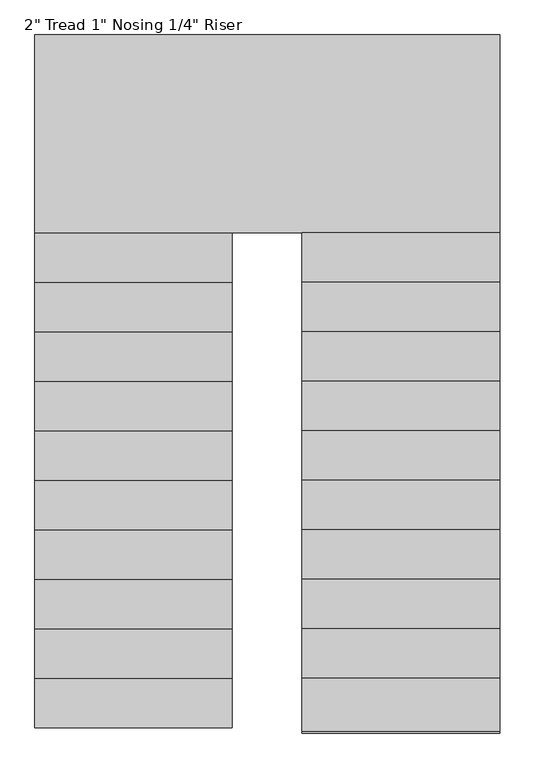
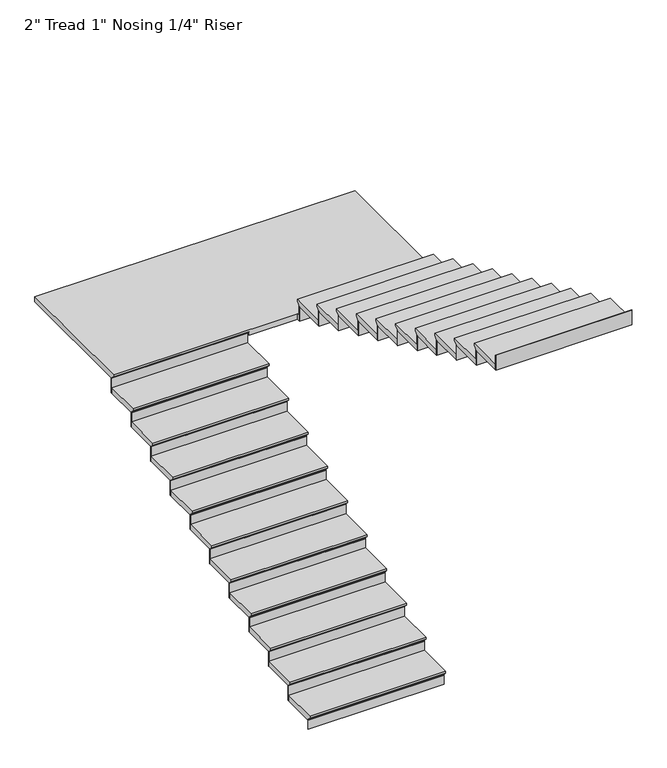
"""IFC4 building model written with IfcOpenShell, lengths in millimetres: stair flight geometry."""

from ifc_helpers import new_model, si_unit, origin, place, context, project, spatial, faceted_brep, source, transform, mapped, element, save


def stair_flight_447a52d2(model_context):
    return source(origin(), model_context, "Body", "Brep", [
        faceted_brep([(-629.5987998, 3364.6067329, 25722.6954545), (-629.5987998, 3364.6067329, 25741.7454545), (-1845.5417538, 3364.6067329, 25741.7454545), (-1845.5417538, 3364.6067329, 25722.6954545), (-629.5987998, 3390.0067329, 25697.2954545), (-1845.5417538, 3390.0067329, 25697.2954545), (-629.5987998, 3694.8067329, 25741.7454545), (-1845.5417538, 3694.8067329, 25741.7454545), (-1845.5417538, 3390.0067329, 25690.9454545), (-1845.5417538, 3694.8067329, 25690.9454545), (-629.5987998, 3694.8067329, 25690.9454545), (-629.5987998, 3390.0067329, 25690.9454545)], [[[0, 1, 2, 3]], [[4, 0, 3, 5]], [[2, 1, 6, 7]], [[8, 9, 10, 11]], [[2, 7, 9, 8, 5, 3]], [[8, 11, 4, 5]], [[6, 1, 0, 4, 11, 10]], [[7, 6, 10, 9]]]),
        faceted_brep([(-629.5987998, 3390.0067329, 25690.9454545), (-629.5987998, 3390.0067329, 25603.2), (-629.5987998, 3396.3567329, 25603.2), (-629.5987998, 3396.3567329, 25690.9454545), (-1845.5417538, 3390.0067329, 25690.9454545), (-1845.5417538, 3396.3567329, 25690.9454545), (-1845.5417538, 3396.3567329, 25603.2), (-1845.5417538, 3390.0067329, 25603.2)], [[[0, 1, 2, 3]], [[4, 5, 6, 7]], [[1, 0, 4, 7]], [[2, 1, 7, 6]], [[3, 2, 6, 5]], [[0, 3, 5, 4]]]),
        faceted_brep([(-629.5987998, 3694.8067329, 25829.4909091), (-629.5987998, 3694.8067329, 25690.9454545), (-629.5987998, 3701.1567329, 25690.9454545), (-629.5987998, 3701.1567329, 25829.4909091), (-1845.5417538, 3694.8067329, 25829.4909091), (-1845.5417538, 3701.1567329, 25829.4909091), (-1845.5417538, 3701.1567329, 25690.9454545), (-1845.5417538, 3694.8067329, 25690.9454545)], [[[0, 1, 2, 3]], [[4, 5, 6, 7]], [[1, 0, 4, 7]], [[2, 1, 7, 6]], [[3, 2, 6, 5]], [[0, 3, 5, 4]]]),
        faceted_brep([(-1845.5417538, 3669.4067329, 25880.2909091), (-629.5987998, 3669.4067329, 25880.2909091), (-629.5987998, 3999.6067329, 25880.2909091), (-1845.5417538, 3999.6067329, 25880.2909091), (-1845.5417538, 3694.8067329, 25829.4909091), (-1845.5417538, 3999.6067329, 25829.4909091), (-629.5987998, 3999.6067329, 25829.4909091), (-629.5987998, 3694.8067329, 25829.4909091), (-1845.5417538, 3694.8067329, 25835.8409091), (-1845.5417538, 3669.4067329, 25861.2409091), (-629.5987998, 3694.8067329, 25835.8409091), (-629.5987998, 3669.4067329, 25861.2409091)], [[[0, 1, 2, 3]], [[4, 5, 6, 7]], [[0, 3, 5, 4, 8, 9]], [[4, 7, 10, 8]], [[2, 1, 11, 10, 7, 6]], [[3, 2, 6, 5]], [[11, 1, 0, 9]], [[10, 11, 9, 8]]]),
        faceted_brep([(-629.5987998, 3999.6067329, 25968.0363636), (-629.5987998, 3999.6067329, 25829.4909091), (-629.5987998, 4005.9567329, 25829.4909091), (-629.5987998, 4005.9567329, 25968.0363636), (-1845.5417538, 3999.6067329, 25968.0363636), (-1845.5417538, 4005.9567329, 25968.0363636), (-1845.5417538, 4005.9567329, 25829.4909091), (-1845.5417538, 3999.6067329, 25829.4909091)], [[[0, 1, 2, 3]], [[4, 5, 6, 7]], [[1, 0, 4, 7]], [[2, 1, 7, 6]], [[3, 2, 6, 5]], [[0, 3, 5, 4]]]),
        faceted_brep([(-1845.5417538, 3974.2067329, 26018.8363636), (-629.5987998, 3974.2067329, 26018.8363636), (-629.5987998, 4304.4067329, 26018.8363636), (-1845.5417538, 4304.4067329, 26018.8363636), (-1845.5417538, 3999.6067329, 25968.0363636), (-1845.5417538, 4304.4067329, 25968.0363636), (-629.5987998, 4304.4067329, 25968.0363636), (-629.5987998, 3999.6067329, 25968.0363636), (-1845.5417538, 3999.6067329, 25974.3863636), (-1845.5417538, 3974.2067329, 25999.7863636), (-629.5987998, 3999.6067329, 25974.3863636), (-629.5987998, 3974.2067329, 25999.7863636)], [[[0, 1, 2, 3]], [[4, 5, 6, 7]], [[0, 3, 5, 4, 8, 9]], [[4, 7, 10, 8]], [[2, 1, 11, 10, 7, 6]], [[3, 2, 6, 5]], [[11, 1, 0, 9]], [[10, 11, 9, 8]]]),
        faceted_brep([(-629.5987998, 4304.4067329, 26106.5818182), (-629.5987998, 4304.4067329, 25968.0363636), (-629.5987998, 4310.7567329, 25968.0363636), (-629.5987998, 4310.7567329, 26106.5818182), (-1845.5417538, 4304.4067329, 26106.5818182), (-1845.5417538, 4310.7567329, 26106.5818182), (-1845.5417538, 4310.7567329, 25968.0363636), (-1845.5417538, 4304.4067329, 25968.0363636)], [[[0, 1, 2, 3]], [[4, 5, 6, 7]], [[1, 0, 4, 7]], [[2, 1, 7, 6]], [[3, 2, 6, 5]], [[0, 3, 5, 4]]]),
        faceted_brep([(-1845.5417538, 4279.0067329, 26157.3818182), (-629.5987998, 4279.0067329, 26157.3818182), (-629.5987998, 4609.2067329, 26157.3818182), (-1845.5417538, 4609.2067329, 26157.3818182), (-1845.5417538, 4304.4067329, 26106.5818182), (-1845.5417538, 4609.2067329, 26106.5818182), (-629.5987998, 4609.2067329, 26106.5818182), (-629.5987998, 4304.4067329, 26106.5818182), (-1845.5417538, 4304.4067329, 26112.9318182), (-1845.5417538, 4279.0067329, 26138.3318182), (-629.5987998, 4304.4067329, 26112.9318182), (-629.5987998, 4279.0067329, 26138.3318182)], [[[0, 1, 2, 3]], [[4, 5, 6, 7]], [[0, 3, 5, 4, 8, 9]], [[4, 7, 10, 8]], [[2, 1, 11, 10, 7, 6]], [[3, 2, 6, 5]], [[11, 1, 0, 9]], [[10, 11, 9, 8]]]),
        faceted_brep([(-629.5987998, 4609.2067329, 26245.1272727), (-629.5987998, 4609.2067329, 26106.5818182), (-629.5987998, 4615.5567329, 26106.5818182), (-629.5987998, 4615.5567329, 26245.1272727), (-1845.5417538, 4609.2067329, 26245.1272727), (-1845.5417538, 4615.5567329, 26245.1272727), (-1845.5417538, 4615.5567329, 26106.5818182), (-1845.5417538, 4609.2067329, 26106.5818182)], [[[0, 1, 2, 3]], [[4, 5, 6, 7]], [[1, 0, 4, 7]], [[2, 1, 7, 6]], [[3, 2, 6, 5]], [[0, 3, 5, 4]]]),
        faceted_brep([(-1845.5417538, 4583.8067329, 26295.9272727), (-629.5987998, 4583.8067329, 26295.9272727), (-629.5987998, 4914.0067329, 26295.9272727), (-1845.5417538, 4914.0067329, 26295.9272727), (-1845.5417538, 4609.2067329, 26245.1272727), (-1845.5417538, 4914.0067329, 26245.1272727), (-629.5987998, 4914.0067329, 26245.1272727), (-629.5987998, 4609.2067329, 26245.1272727), (-1845.5417538, 4609.2067329, 26251.4772727), (-1845.5417538, 4583.8067329, 26276.8772727), (-629.5987998, 4609.2067329, 26251.4772727), (-629.5987998, 4583.8067329, 26276.8772727)], [[[0, 1, 2, 3]], [[4, 5, 6, 7]], [[0, 3, 5, 4, 8, 9]], [[4, 7, 10, 8]], [[2, 1, 11, 10, 7, 6]], [[3, 2, 6, 5]], [[11, 1, 0, 9]], [[10, 11, 9, 8]]]),
        faceted_brep([(-629.5987998, 4914.0067329, 26383.6727273), (-629.5987998, 4914.0067329, 26245.1272727), (-629.5987998, 4920.3567329, 26245.1272727), (-629.5987998, 4920.3567329, 26383.6727273), (-1845.5417538, 4914.0067329, 26383.6727273), (-1845.5417538, 4920.3567329, 26383.6727273), (-1845.5417538, 4920.3567329, 26245.1272727), (-1845.5417538, 4914.0067329, 26245.1272727)], [[[0, 1, 2, 3]], [[4, 5, 6, 7]], [[1, 0, 4, 7]], [[2, 1, 7, 6]], [[3, 2, 6, 5]], [[0, 3, 5, 4]]]),
        faceted_brep([(-1845.5417538, 4888.6067329, 26434.4727273), (-629.5987998, 4888.6067329, 26434.4727273), (-629.5987998, 5218.8067329, 26434.4727273), (-1845.5417538, 5218.8067329, 26434.4727273), (-1845.5417538, 4914.0067329, 26383.6727273), (-1845.5417538, 5218.8067329, 26383.6727273), (-629.5987998, 5218.8067329, 26383.6727273), (-629.5987998, 4914.0067329, 26383.6727273), (-1845.5417538, 4914.0067329, 26390.0227273), (-1845.5417538, 4888.6067329, 26415.4227273), (-629.5987998, 4914.0067329, 26390.0227273), (-629.5987998, 4888.6067329, 26415.4227273)], [[[0, 1, 2, 3]], [[4, 5, 6, 7]], [[0, 3, 5, 4, 8, 9]], [[4, 7, 10, 8]], [[2, 1, 11, 10, 7, 6]], [[3, 2, 6, 5]], [[11, 1, 0, 9]], [[10, 11, 9, 8]]]),
        faceted_brep([(-629.5987998, 5218.8067329, 26522.2181818), (-629.5987998, 5218.8067329, 26383.6727273), (-629.5987998, 5225.1567329, 26383.6727273), (-629.5987998, 5225.1567329, 26522.2181818), (-1845.5417538, 5218.8067329, 26522.2181818), (-1845.5417538, 5225.1567329, 26522.2181818), (-1845.5417538, 5225.1567329, 26383.6727273), (-1845.5417538, 5218.8067329, 26383.6727273)], [[[0, 1, 2, 3]], [[4, 5, 6, 7]], [[1, 0, 4, 7]], [[2, 1, 7, 6]], [[3, 2, 6, 5]], [[0, 3, 5, 4]]]),
        faceted_brep([(-1845.5417538, 5193.4067329, 26573.0181818), (-629.5987998, 5193.4067329, 26573.0181818), (-629.5987998, 5523.6067329, 26573.0181818), (-1845.5417538, 5523.6067329, 26573.0181818), (-1845.5417538, 5218.8067329, 26522.2181818), (-1845.5417538, 5523.6067329, 26522.2181818), (-629.5987998, 5523.6067329, 26522.2181818), (-629.5987998, 5218.8067329, 26522.2181818), (-1845.5417538, 5218.8067329, 26528.5681818), (-1845.5417538, 5193.4067329, 26553.9681818), (-629.5987998, 5218.8067329, 26528.5681818), (-629.5987998, 5193.4067329, 26553.9681818)], [[[0, 1, 2, 3]], [[4, 5, 6, 7]], [[0, 3, 5, 4, 8, 9]], [[4, 7, 10, 8]], [[2, 1, 11, 10, 7, 6]], [[3, 2, 6, 5]], [[11, 1, 0, 9]], [[10, 11, 9, 8]]]),
        faceted_brep([(-629.5987998, 5523.6067329, 26660.7636364), (-629.5987998, 5523.6067329, 26522.2181818), (-629.5987998, 5529.9567329, 26522.2181818), (-629.5987998, 5529.9567329, 26660.7636364), (-1845.5417538, 5523.6067329, 26660.7636364), (-1845.5417538, 5529.9567329, 26660.7636364), (-1845.5417538, 5529.9567329, 26522.2181818), (-1845.5417538, 5523.6067329, 26522.2181818)], [[[0, 1, 2, 3]], [[4, 5, 6, 7]], [[1, 0, 4, 7]], [[2, 1, 7, 6]], [[3, 2, 6, 5]], [[0, 3, 5, 4]]]),
        faceted_brep([(-1845.5417538, 5498.2067329, 26711.5636364), (-629.5987998, 5498.2067329, 26711.5636364), (-629.5987998, 5828.4067329, 26711.5636364), (-1845.5417538, 5828.4067329, 26711.5636364), (-1845.5417538, 5523.6067329, 26660.7636364), (-1845.5417538, 5828.4067329, 26660.7636364), (-629.5987998, 5828.4067329, 26660.7636364), (-629.5987998, 5523.6067329, 26660.7636364), (-1845.5417538, 5523.6067329, 26667.1136364), (-1845.5417538, 5498.2067329, 26692.5136364), (-629.5987998, 5523.6067329, 26667.1136364), (-629.5987998, 5498.2067329, 26692.5136364)], [[[0, 1, 2, 3]], [[4, 5, 6, 7]], [[0, 3, 5, 4, 8, 9]], [[4, 7, 10, 8]], [[2, 1, 11, 10, 7, 6]], [[3, 2, 6, 5]], [[11, 1, 0, 9]], [[10, 11, 9, 8]]]),
        faceted_brep([(-629.5987998, 5828.4067329, 26799.3090909), (-629.5987998, 5828.4067329, 26660.7636364), (-629.5987998, 5834.7567329, 26660.7636364), (-629.5987998, 5834.7567329, 26799.3090909), (-1845.5417538, 5828.4067329, 26799.3090909), (-1845.5417538, 5834.7567329, 26799.3090909), (-1845.5417538, 5834.7567329, 26660.7636364), (-1845.5417538, 5828.4067329, 26660.7636364)], [[[0, 1, 2, 3]], [[4, 5, 6, 7]], [[1, 0, 4, 7]], [[2, 1, 7, 6]], [[3, 2, 6, 5]], [[0, 3, 5, 4]]]),
        faceted_brep([(-1845.5417538, 5803.0067329, 26850.1090909), (-629.5987998, 5803.0067329, 26850.1090909), (-629.5987998, 6133.2067329, 26850.1090909), (-1845.5417538, 6133.2067329, 26850.1090909), (-1845.5417538, 5828.4067329, 26799.3090909), (-1845.5417538, 6133.2067329, 26799.3090909), (-629.5987998, 6133.2067329, 26799.3090909), (-629.5987998, 5828.4067329, 26799.3090909), (-1845.5417538, 5828.4067329, 26805.6590909), (-1845.5417538, 5803.0067329, 26831.0590909), (-629.5987998, 5828.4067329, 26805.6590909), (-629.5987998, 5803.0067329, 26831.0590909)], [[[0, 1, 2, 3]], [[4, 5, 6, 7]], [[0, 3, 5, 4, 8, 9]], [[4, 7, 10, 8]], [[2, 1, 11, 10, 7, 6]], [[3, 2, 6, 5]], [[11, 1, 0, 9]], [[10, 11, 9, 8]]]),
        faceted_brep([(-629.5987998, 6133.2067329, 26937.8545455), (-629.5987998, 6133.2067329, 26799.3090909), (-629.5987998, 6139.5567329, 26799.3090909), (-629.5987998, 6139.5567329, 26937.8545455), (-1845.5417538, 6133.2067329, 26937.8545455), (-1845.5417538, 6139.5567329, 26937.8545455), (-1845.5417538, 6139.5567329, 26799.3090909), (-1845.5417538, 6133.2067329, 26799.3090909)], [[[0, 1, 2, 3]], [[4, 5, 6, 7]], [[1, 0, 4, 7]], [[2, 1, 7, 6]], [[3, 2, 6, 5]], [[0, 3, 5, 4]]]),
        faceted_brep([(-1845.5417538, 6107.8067329, 26988.6545455), (-629.5987998, 6107.8067329, 26988.6545455), (-629.5987998, 6438.0067329, 26988.6545455), (-1845.5417538, 6438.0067329, 26988.6545455), (-1845.5417538, 6133.2067329, 26937.8545455), (-1845.5417538, 6438.0067329, 26937.8545455), (-629.5987998, 6438.0067329, 26937.8545455), (-629.5987998, 6133.2067329, 26937.8545455), (-1845.5417538, 6133.2067329, 26944.2045455), (-1845.5417538, 6107.8067329, 26969.6045455), (-629.5987998, 6133.2067329, 26944.2045455), (-629.5987998, 6107.8067329, 26969.6045455)], [[[0, 1, 2, 3]], [[4, 5, 6, 7]], [[0, 3, 5, 4, 8, 9]], [[4, 7, 10, 8]], [[2, 1, 11, 10, 7, 6]], [[3, 2, 6, 5]], [[11, 1, 0, 9]], [[10, 11, 9, 8]]]),
        faceted_brep([(-629.5987998, 6438.0067329, 27076.4), (-629.5987998, 6438.0067329, 26937.8545455), (-629.5987998, 6444.3567329, 26937.8545455), (-629.5987998, 6444.3567329, 27076.4), (-1845.5417538, 6438.0067329, 27076.4), (-1845.5417538, 6444.3567329, 27076.4), (-1845.5417538, 6444.3567329, 26937.8545455), (-1845.5417538, 6438.0067329, 26937.8545455)], [[[0, 1, 2, 3]], [[4, 5, 6, 7]], [[1, 0, 4, 7]], [[2, 1, 7, 6]], [[3, 2, 6, 5]], [[0, 3, 5, 4]]]),
        faceted_brep([(1021.4012085, 6387.2067329, 27127.2), (1021.4012085, 7631.8067329, 27127.2), (-1845.5417538, 7631.8067329, 27127.2), (-1845.5417538, 6412.6067329, 27127.2), (-197.7987915, 6412.6067329, 27127.2), (-197.7987915, 6387.2067329, 27127.2), (1021.4012085, 7631.8067329, 27076.4), (1021.4012085, 6387.2067329, 27076.4), (-197.7987915, 6387.2067329, 27076.4), (-197.7987915, 6412.6067329, 27076.4), (-629.5987998, 6412.6067329, 27076.4), (-629.5987998, 6438.0067329, 27076.4), (-1845.5417538, 6438.0067329, 27076.4), (-1845.5417538, 7631.8067329, 27076.4), (-629.5987998, 6438.0067329, 27082.75), (-1845.5417538, 6438.0067329, 27082.75), (-1845.5417538, 6412.6067329, 27108.15), (-629.5987998, 6412.6067329, 27108.15)], [[[0, 1, 2, 3, 4, 5]], [[6, 7, 8, 9, 10, 11, 12, 13]], [[1, 0, 7, 6]], [[2, 1, 6, 13]], [[12, 11, 14, 15]], [[4, 3, 16, 17, 10, 9]], [[5, 4, 9, 8]], [[0, 5, 8, 7]], [[16, 15, 14, 17]], [[3, 2, 13, 12, 15, 16]], [[11, 10, 17, 14]]]),
        faceted_brep([(-197.7987915, 6387.2067329, 27214.9454545), (-197.7987915, 6387.2067329, 27076.4), (-197.7987915, 6380.8567329, 27076.4), (-197.7987915, 6380.8567329, 27214.9454545), (1021.4012085, 6387.2067329, 27214.9454545), (1021.4012085, 6380.8567329, 27214.9454545), (1021.4012085, 6380.8567329, 27076.4), (1021.4012085, 6387.2067329, 27076.4)], [[[0, 1, 2, 3]], [[4, 5, 6, 7]], [[1, 0, 4, 7]], [[2, 1, 7, 6]], [[3, 2, 6, 5]], [[0, 3, 5, 4]]]),
        faceted_brep([(1021.4012085, 6412.6067329, 27265.7454545), (-197.7987915, 6412.6067329, 27265.7454545), (-197.7987915, 6082.4067329, 27265.7454545), (1021.4012085, 6082.4067329, 27265.7454545), (1021.4012085, 6387.2067329, 27214.9454545), (1021.4012085, 6082.4067329, 27214.9454545), (-197.7987915, 6082.4067329, 27214.9454545), (-197.7987915, 6387.2067329, 27214.9454545), (1021.4012085, 6387.2067329, 27221.2954545), (1021.4012085, 6412.6067329, 27246.6954545), (-197.7987915, 6387.2067329, 27221.2954545), (-197.7987915, 6412.6067329, 27246.6954545)], [[[0, 1, 2, 3]], [[4, 5, 6, 7]], [[0, 3, 5, 4, 8, 9]], [[4, 7, 10, 8]], [[2, 1, 11, 10, 7, 6]], [[3, 2, 6, 5]], [[11, 1, 0, 9]], [[10, 11, 9, 8]]]),
        faceted_brep([(-197.7987915, 6082.4067329, 27353.4909091), (-197.7987915, 6082.4067329, 27214.9454545), (-197.7987915, 6076.0567329, 27214.9454545), (-197.7987915, 6076.0567329, 27353.4909091), (1021.4012085, 6082.4067329, 27353.4909091), (1021.4012085, 6076.0567329, 27353.4909091), (1021.4012085, 6076.0567329, 27214.9454545), (1021.4012085, 6082.4067329, 27214.9454545)], [[[0, 1, 2, 3]], [[4, 5, 6, 7]], [[1, 0, 4, 7]], [[2, 1, 7, 6]], [[3, 2, 6, 5]], [[0, 3, 5, 4]]]),
        faceted_brep([(1021.4012085, 6107.8067329, 27404.2909091), (-197.7987915, 6107.8067329, 27404.2909091), (-197.7987915, 5777.6067329, 27404.2909091), (1021.4012085, 5777.6067329, 27404.2909091), (1021.4012085, 6082.4067329, 27353.4909091), (1021.4012085, 5777.6067329, 27353.4909091), (-197.7987915, 5777.6067329, 27353.4909091), (-197.7987915, 6082.4067329, 27353.4909091), (1021.4012085, 6082.4067329, 27359.8409091), (1021.4012085, 6107.8067329, 27385.2409091), (-197.7987915, 6082.4067329, 27359.8409091), (-197.7987915, 6107.8067329, 27385.2409091)], [[[0, 1, 2, 3]], [[4, 5, 6, 7]], [[0, 3, 5, 4, 8, 9]], [[4, 7, 10, 8]], [[2, 1, 11, 10, 7, 6]], [[3, 2, 6, 5]], [[11, 1, 0, 9]], [[10, 11, 9, 8]]]),
        faceted_brep([(-197.7987915, 5777.6067329, 27492.0363636), (-197.7987915, 5777.6067329, 27353.4909091), (-197.7987915, 5771.2567329, 27353.4909091), (-197.7987915, 5771.2567329, 27492.0363636), (1021.4012085, 5777.6067329, 27492.0363636), (1021.4012085, 5771.2567329, 27492.0363636), (1021.4012085, 5771.2567329, 27353.4909091), (1021.4012085, 5777.6067329, 27353.4909091)], [[[0, 1, 2, 3]], [[4, 5, 6, 7]], [[1, 0, 4, 7]], [[2, 1, 7, 6]], [[3, 2, 6, 5]], [[0, 3, 5, 4]]]),
        faceted_brep([(1021.4012085, 5803.0067329, 27542.8363636), (-197.7987915, 5803.0067329, 27542.8363636), (-197.7987915, 5472.8067329, 27542.8363636), (1021.4012085, 5472.8067329, 27542.8363636), (1021.4012085, 5777.6067329, 27492.0363636), (1021.4012085, 5472.8067329, 27492.0363636), (-197.7987915, 5472.8067329, 27492.0363636), (-197.7987915, 5777.6067329, 27492.0363636), (1021.4012085, 5777.6067329, 27498.3863636), (1021.4012085, 5803.0067329, 27523.7863636), (-197.7987915, 5777.6067329, 27498.3863636), (-197.7987915, 5803.0067329, 27523.7863636)], [[[0, 1, 2, 3]], [[4, 5, 6, 7]], [[0, 3, 5, 4, 8, 9]], [[4, 7, 10, 8]], [[2, 1, 11, 10, 7, 6]], [[3, 2, 6, 5]], [[11, 1, 0, 9]], [[10, 11, 9, 8]]]),
        faceted_brep([(-197.7987915, 5472.8067329, 27630.5818182), (-197.7987915, 5472.8067329, 27492.0363636), (-197.7987915, 5466.4567329, 27492.0363636), (-197.7987915, 5466.4567329, 27630.5818182), (1021.4012085, 5472.8067329, 27630.5818182), (1021.4012085, 5466.4567329, 27630.5818182), (1021.4012085, 5466.4567329, 27492.0363636), (1021.4012085, 5472.8067329, 27492.0363636)], [[[0, 1, 2, 3]], [[4, 5, 6, 7]], [[1, 0, 4, 7]], [[2, 1, 7, 6]], [[3, 2, 6, 5]], [[0, 3, 5, 4]]]),
        faceted_brep([(1021.4012085, 5498.2067329, 27681.3818182), (-197.7987915, 5498.2067329, 27681.3818182), (-197.7987915, 5168.0067329, 27681.3818182), (1021.4012085, 5168.0067329, 27681.3818182), (1021.4012085, 5472.8067329, 27630.5818182), (1021.4012085, 5168.0067329, 27630.5818182), (-197.7987915, 5168.0067329, 27630.5818182), (-197.7987915, 5472.8067329, 27630.5818182), (1021.4012085, 5472.8067329, 27636.9318182), (1021.4012085, 5498.2067329, 27662.3318182), (-197.7987915, 5472.8067329, 27636.9318182), (-197.7987915, 5498.2067329, 27662.3318182)], [[[0, 1, 2, 3]], [[4, 5, 6, 7]], [[0, 3, 5, 4, 8, 9]], [[4, 7, 10, 8]], [[2, 1, 11, 10, 7, 6]], [[3, 2, 6, 5]], [[11, 1, 0, 9]], [[10, 11, 9, 8]]]),
        faceted_brep([(-197.7987915, 5168.0067329, 27769.1272727), (-197.7987915, 5168.0067329, 27630.5818182), (-197.7987915, 5161.6567329, 27630.5818182), (-197.7987915, 5161.6567329, 27769.1272727), (1021.4012085, 5168.0067329, 27769.1272727), (1021.4012085, 5161.6567329, 27769.1272727), (1021.4012085, 5161.6567329, 27630.5818182), (1021.4012085, 5168.0067329, 27630.5818182)], [[[0, 1, 2, 3]], [[4, 5, 6, 7]], [[1, 0, 4, 7]], [[2, 1, 7, 6]], [[3, 2, 6, 5]], [[0, 3, 5, 4]]]),
        faceted_brep([(1021.4012085, 5193.4067329, 27819.9272727), (-197.7987915, 5193.4067329, 27819.9272727), (-197.7987915, 4863.2067329, 27819.9272727), (1021.4012085, 4863.2067329, 27819.9272727), (1021.4012085, 5168.0067329, 27769.1272727), (1021.4012085, 4863.2067329, 27769.1272727), (-197.7987915, 4863.2067329, 27769.1272727), (-197.7987915, 5168.0067329, 27769.1272727), (1021.4012085, 5168.0067329, 27775.4772727), (1021.4012085, 5193.4067329, 27800.8772727), (-197.7987915, 5168.0067329, 27775.4772727), (-197.7987915, 5193.4067329, 27800.8772727)], [[[0, 1, 2, 3]], [[4, 5, 6, 7]], [[0, 3, 5, 4, 8, 9]], [[4, 7, 10, 8]], [[2, 1, 11, 10, 7, 6]], [[3, 2, 6, 5]], [[11, 1, 0, 9]], [[10, 11, 9, 8]]]),
        faceted_brep([(-197.7987915, 4863.2067329, 27907.6727273), (-197.7987915, 4863.2067329, 27769.1272727), (-197.7987915, 4856.8567329, 27769.1272727), (-197.7987915, 4856.8567329, 27907.6727273), (1021.4012085, 4863.2067329, 27907.6727273), (1021.4012085, 4856.8567329, 27907.6727273), (1021.4012085, 4856.8567329, 27769.1272727), (1021.4012085, 4863.2067329, 27769.1272727)], [[[0, 1, 2, 3]], [[4, 5, 6, 7]], [[1, 0, 4, 7]], [[2, 1, 7, 6]], [[3, 2, 6, 5]], [[0, 3, 5, 4]]]),
        faceted_brep([(1021.4012085, 4888.6067329, 27958.4727273), (-197.7987915, 4888.6067329, 27958.4727273), (-197.7987915, 4558.4067329, 27958.4727273), (1021.4012085, 4558.4067329, 27958.4727273), (1021.4012085, 4863.2067329, 27907.6727273), (1021.4012085, 4558.4067329, 27907.6727273), (-197.7987915, 4558.4067329, 27907.6727273), (-197.7987915, 4863.2067329, 27907.6727273), (1021.4012085, 4863.2067329, 27914.0227273), (1021.4012085, 4888.6067329, 27939.4227273), (-197.7987915, 4863.2067329, 27914.0227273), (-197.7987915, 4888.6067329, 27939.4227273)], [[[0, 1, 2, 3]], [[4, 5, 6, 7]], [[0, 3, 5, 4, 8, 9]], [[4, 7, 10, 8]], [[2, 1, 11, 10, 7, 6]], [[3, 2, 6, 5]], [[11, 1, 0, 9]], [[10, 11, 9, 8]]]),
        faceted_brep([(-197.7987915, 4558.4067329, 28046.2181818), (-197.7987915, 4558.4067329, 27907.6727273), (-197.7987915, 4552.0567329, 27907.6727273), (-197.7987915, 4552.0567329, 28046.2181818), (1021.4012085, 4558.4067329, 28046.2181818), (1021.4012085, 4552.0567329, 28046.2181818), (1021.4012085, 4552.0567329, 27907.6727273), (1021.4012085, 4558.4067329, 27907.6727273)], [[[0, 1, 2, 3]], [[4, 5, 6, 7]], [[1, 0, 4, 7]], [[2, 1, 7, 6]], [[3, 2, 6, 5]], [[0, 3, 5, 4]]]),
        faceted_brep([(1021.4012085, 4583.8067329, 28097.0181818), (-197.7987915, 4583.8067329, 28097.0181818), (-197.7987915, 4253.6067329, 28097.0181818), (1021.4012085, 4253.6067329, 28097.0181818), (1021.4012085, 4558.4067329, 28046.2181818), (1021.4012085, 4253.6067329, 28046.2181818), (-197.7987915, 4253.6067329, 28046.2181818), (-197.7987915, 4558.4067329, 28046.2181818), (1021.4012085, 4558.4067329, 28052.5681818), (1021.4012085, 4583.8067329, 28077.9681818), (-197.7987915, 4558.4067329, 28052.5681818), (-197.7987915, 4583.8067329, 28077.9681818)], [[[0, 1, 2, 3]], [[4, 5, 6, 7]], [[0, 3, 5, 4, 8, 9]], [[4, 7, 10, 8]], [[2, 1, 11, 10, 7, 6]], [[3, 2, 6, 5]], [[11, 1, 0, 9]], [[10, 11, 9, 8]]]),
        faceted_brep([(-197.7987915, 4253.6067329, 28184.7636364), (-197.7987915, 4253.6067329, 28046.2181818), (-197.7987915, 4247.2567329, 28046.2181818), (-197.7987915, 4247.2567329, 28184.7636364), (1021.4012085, 4253.6067329, 28184.7636364), (1021.4012085, 4247.2567329, 28184.7636364), (1021.4012085, 4247.2567329, 28046.2181818), (1021.4012085, 4253.6067329, 28046.2181818)], [[[0, 1, 2, 3]], [[4, 5, 6, 7]], [[1, 0, 4, 7]], [[2, 1, 7, 6]], [[3, 2, 6, 5]], [[0, 3, 5, 4]]]),
        faceted_brep([(1021.4012085, 4279.0067329, 28235.5636364), (-197.7987915, 4279.0067329, 28235.5636364), (-197.7987915, 3948.8067329, 28235.5636364), (1021.4012085, 3948.8067329, 28235.5636364), (1021.4012085, 4253.6067329, 28184.7636364), (1021.4012085, 3948.8067329, 28184.7636364), (-197.7987915, 3948.8067329, 28184.7636364), (-197.7987915, 4253.6067329, 28184.7636364), (1021.4012085, 4253.6067329, 28191.1136364), (1021.4012085, 4279.0067329, 28216.5136364), (-197.7987915, 4253.6067329, 28191.1136364), (-197.7987915, 4279.0067329, 28216.5136364)], [[[0, 1, 2, 3]], [[4, 5, 6, 7]], [[0, 3, 5, 4, 8, 9]], [[4, 7, 10, 8]], [[2, 1, 11, 10, 7, 6]], [[3, 2, 6, 5]], [[11, 1, 0, 9]], [[10, 11, 9, 8]]]),
        faceted_brep([(-197.7987915, 3948.8067329, 28323.3090909), (-197.7987915, 3948.8067329, 28184.7636364), (-197.7987915, 3942.4567329, 28184.7636364), (-197.7987915, 3942.4567329, 28323.3090909), (1021.4012085, 3948.8067329, 28323.3090909), (1021.4012085, 3942.4567329, 28323.3090909), (1021.4012085, 3942.4567329, 28184.7636364), (1021.4012085, 3948.8067329, 28184.7636364)], [[[0, 1, 2, 3]], [[4, 5, 6, 7]], [[1, 0, 4, 7]], [[2, 1, 7, 6]], [[3, 2, 6, 5]], [[0, 3, 5, 4]]]),
        faceted_brep([(1021.4012085, 3974.2067329, 28374.1090909), (-197.7987915, 3974.2067329, 28374.1090909), (-197.7987915, 3644.0067329, 28374.1090909), (1021.4012085, 3644.0067329, 28374.1090909), (1021.4012085, 3948.8067329, 28323.3090909), (1021.4012085, 3644.0067329, 28323.3090909), (-197.7987915, 3644.0067329, 28323.3090909), (-197.7987915, 3948.8067329, 28323.3090909), (1021.4012085, 3948.8067329, 28329.6590909), (1021.4012085, 3974.2067329, 28355.0590909), (-197.7987915, 3948.8067329, 28329.6590909), (-197.7987915, 3974.2067329, 28355.0590909)], [[[0, 1, 2, 3]], [[4, 5, 6, 7]], [[0, 3, 5, 4, 8, 9]], [[4, 7, 10, 8]], [[2, 1, 11, 10, 7, 6]], [[3, 2, 6, 5]], [[11, 1, 0, 9]], [[10, 11, 9, 8]]]),
        faceted_brep([(-197.7987915, 3644.0067329, 28461.8545455), (-197.7987915, 3644.0067329, 28323.3090909), (-197.7987915, 3637.6567329, 28323.3090909), (-197.7987915, 3637.6567329, 28461.8545455), (1021.4012085, 3644.0067329, 28461.8545455), (1021.4012085, 3637.6567329, 28461.8545455), (1021.4012085, 3637.6567329, 28323.3090909), (1021.4012085, 3644.0067329, 28323.3090909)], [[[0, 1, 2, 3]], [[4, 5, 6, 7]], [[1, 0, 4, 7]], [[2, 1, 7, 6]], [[3, 2, 6, 5]], [[0, 3, 5, 4]]]),
        faceted_brep([(-197.7987915, 3339.2067329, 28600.4), (-197.7987915, 3339.2067329, 28461.8545455), (-197.7987915, 3332.8567329, 28461.8545455), (-197.7987915, 3332.8567329, 28600.4), (1021.4012085, 3339.2067329, 28600.4), (1021.4012085, 3332.8567329, 28600.4), (1021.4012085, 3332.8567329, 28461.8545455), (1021.4012085, 3339.2067329, 28461.8545455)], [[[0, 1, 2, 3]], [[4, 5, 6, 7]], [[1, 0, 4, 7]], [[2, 1, 7, 6]], [[3, 2, 6, 5]], [[0, 3, 5, 4]]]),
        faceted_brep([(1021.4012085, 3669.4067329, 28512.6545455), (-197.7987915, 3669.4067329, 28512.6545455), (-197.7987915, 3339.2067329, 28512.6545455), (1021.4012085, 3339.2067329, 28512.6545455), (1021.4012085, 3644.0067329, 28461.8545455), (1021.4012085, 3339.2067329, 28461.8545455), (-197.7987915, 3339.2067329, 28461.8545455), (-197.7987915, 3644.0067329, 28461.8545455), (1021.4012085, 3644.0067329, 28468.2045455), (1021.4012085, 3669.4067329, 28493.6045455), (-197.7987915, 3644.0067329, 28468.2045455), (-197.7987915, 3669.4067329, 28493.6045455)], [[[0, 1, 2, 3]], [[4, 5, 6, 7]], [[0, 3, 5, 4, 8, 9]], [[4, 7, 10, 8]], [[2, 1, 11, 10, 7, 6]], [[3, 2, 6, 5]], [[11, 1, 0, 9]], [[10, 11, 9, 8]]]),
    ])


if __name__ == "__main__":
    model = new_model("IFC4")
    model_context = context("Model", 3, world=origin())
    ifc_project = project(units=[si_unit("LENGTHUNIT", "METRE", prefix="MILLI")], contexts=[model_context])
    site = spatial("IfcSite", under=ifc_project)
    building = spatial("IfcBuilding", under=site)
    placement = place(None, origin())
    stair_flight_shape = stair_flight_447a52d2(model_context)
    element("IfcStairFlight", 1, ObjectType="2\" Tread 1\" Nosing 1/4\" Riser", at=placement, inside=building, context=model_context, shape_type="MappedRepresentation", body=[
        mapped(stair_flight_shape, transform((0.0, 0.0, 0.0), x_axis=(1.0, 0.0, 0.0), y_axis=(0.0, 1.0, 0.0), z_axis=(0.0, 0.0, 1.0))),
    ])
    save(model, "model.ifc")
